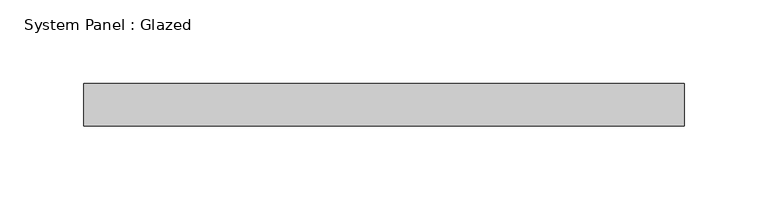
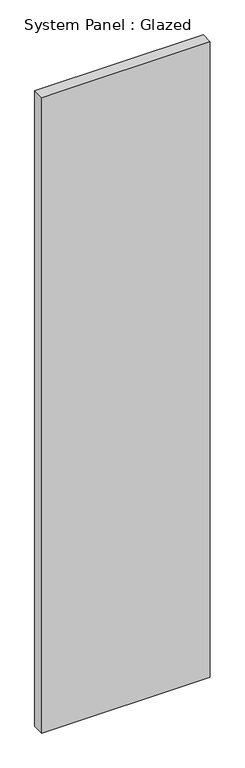
"""IFC4 building model written with IfcOpenShell, lengths in millimetres: plate geometry, System Panel : Glazed."""

from ifc_helpers import new_model, si_unit, origin, origin_with_axes, place, context, project, spatial, polyline, outline, extrude, source, transform, mapped, element, save


def system_panel_glazed_76557058(model_context):
    return source(origin(), model_context, "Body", "SweptSolid", [
        extrude(outline(polyline([(179.3875, 19.05), (-179.3875, 19.05), (-179.3875, 44.45), (179.3875, 44.45), (179.3875, 19.05)])), origin_with_axes(), (0.0, 0.0, 1.0), 1429.7181357),
    ])


if __name__ == "__main__":
    model = new_model("IFC4")
    model_context = context("Model", 3, world=origin())
    ifc_project = project(units=[si_unit("LENGTHUNIT", "METRE", prefix="MILLI")], contexts=[model_context])
    site = spatial("IfcSite", under=ifc_project)
    building = spatial("IfcBuilding", under=site)
    placement = place(None, origin())
    system_panel_glazed_shape = system_panel_glazed_76557058(model_context)
    element("IfcPlate", 1, ObjectType="System Panel : Glazed", at=placement, inside=building, context=model_context, shape_type="MappedRepresentation", body=[
        mapped(system_panel_glazed_shape, transform((0.0, 0.0, 0.0), x_axis=(1.0, 0.0, 0.0), y_axis=(0.0, 1.0, 0.0), z_axis=(0.0, 0.0, 1.0))),
    ])
    save(model, "model.ifc")

# Revit data of these elements
# Type "System Panel : Glazed"
#   Construction Type Id = "GSP4R"
#   Analytic Construction = "1/8 in Pilkington single glazing"
#   Visual Light Transmittance = 0.9
#   Solar Heat Gain Coefficient = 0.86
#   Heat Transfer Coefficient (U) = 1.18115 BTU/(h·ft²·°F)
#   Define Thermal Properties by = 1
# Element 1 (IfcPlate, "System Panel : Glazed")
#   Materials on its faces: "Glass"
# Materials
#   "Glass": class "Glass", colour RGB 0 128 192, transparency 0.75, Description = "Soda Lime Glass", Cost = 0
